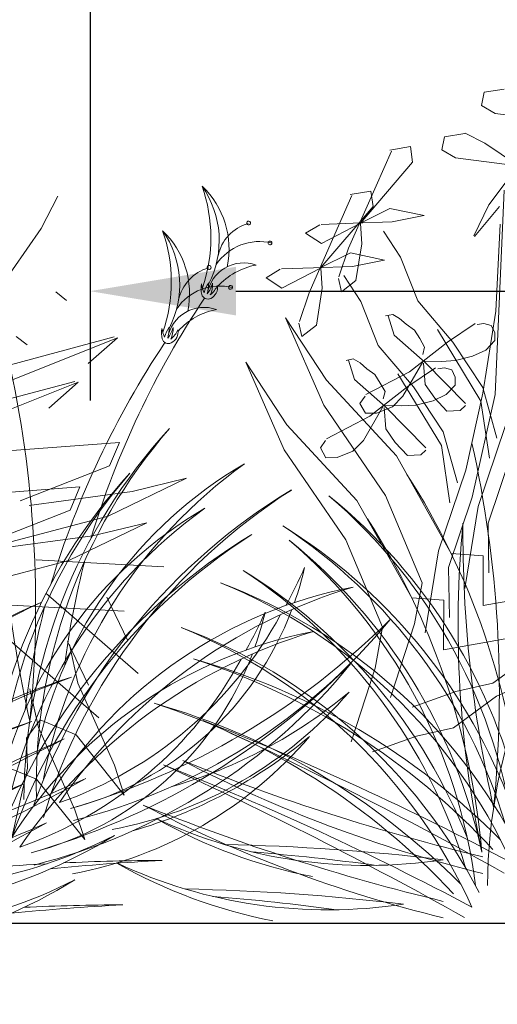
# Model space of a CAD drawing. Units: inches. Extents: x 89 to 490, y -59 to 378.
# Tile 5 of 20: x 326 to 339, y -26 to 1. Entities that reach past the tile are written whole.
import ezdxf

# ---------------------------------------------------------------- set-up
doc = ezdxf.new("R2010")
doc.units = ezdxf.units.IN
doc.header["$MEASUREMENT"] = 0
for name, color, linetype, lineweight in [('A-ANNO-DIMS', 2, 'Continuous', 18), ('L-PLNT', 94, 'Continuous', 18), ('L-PLNT-EDGE', 31, 'Continuous', 25)]:
    doc.layers.add(name, color=color, linetype=linetype, lineweight=lineweight)
doc.layers.add('fl', color=73, linetype='Continuous', lineweight=9, true_color=0xa3d166)
doc.styles.get("Standard").update_dxf_attribs({"font": 'arial.ttf'})
doc.dimstyles.get("Standard").update_dxf_attribs({"dimtxt": 6, "dimasz": 4, "dimexe": 3, "dimexo": 3, "dimgap": 0.09, "dimtad": 0, "dimtih": 1, "dimtoh": 1, "dimdec": 1, "dimzin": 0, "dimdsep": 46, "dimlunit": 3, "dimtxsty": 'Standard', "dimcen": 0.09, "dimadec": 0, "dimazin": 0, "dimtfac": 1, "dimtdec": 1, "dimtofl": 0, "dimtmove": 0, "dimatfit": 3, "dimfxl": 1, "dimtolj": 1, "dimtzin": 0, "dimarcsym": 0})

# ---------------------------------------------------------------- blocks, each defined once
blk = doc.blocks.new('Plantation')
at = {"layer": 'fl'}
for p, q in [((562.897, 34.348), (562.341, 34.259)), ((562.341, 34.259), (562.268, 33.899)), ((562.268, 33.899), (562.643, 33.679)), ((562.643, 33.679), (564.267, 33.469)), ((561.257, 33.041), (561.184, 32.681)), ((561.813, 33.13), (561.257, 33.041)), ((561.819, 33.139), (562.363, 32.866)), ((559.759, 32.671), (560.323, 32.769)), ((560.323, 32.769), (560.381, 32.343)), ((561.184, 32.681), (561.559, 32.461)), ((562.363, 32.866), (563.259, 32.265)), ((559.17, 31.216), (559.802, 32.648)), ((561.559, 32.461), (563.183, 32.251)), ((562.47, 31.169), (563.4, 32.416)), ((560.381, 32.343), (558.952, 30.67)), ((562.894, 31.579), (562.65, 25.971)), ((550.656, 31.412), (550.2, 30.521)), ((558.086, 29.998), (558.718, 31.43)), ((558.675, 31.453), (559.239, 31.551)), ((559.239, 31.551), (559.297, 31.125)), ((559.297, 31.125), (557.868, 29.452)), ((558.629, 29.982), (559.17, 31.216)), ((559.762, 31.074), (558.915, 30.657)), ((560.695, 30.877), (559.762, 31.074)), ((562.061, 30.328), (562.47, 31.169)), ((562.075, 30.305), (562.765, 31.127)), ((559.819, 30.704), (560.688, 30.879)), ((550.2, 30.521), (548.393, 27.932)), ((557.835, 30.626), (557.449, 30.393)), ((557.877, 30.637), (558.751, 30.667)), ((557.881, 30.111), (558.94, 30.658)), ((558.751, 30.667), (559.819, 30.704)), ((558.987, 30.105), (558.952, 30.658)), ((562.666, 28.259), (562.78, 30.644)), ((557.449, 30.393), (557.881, 30.111)), ((559.585, 30.453), (560.047, 29.739)), ((557.545, 28.764), (558.086, 29.998)), ((558.364, 29.196), (558.629, 29.982)), ((558.829, 29.096), (558.987, 30.105)), ((558.678, 29.856), (557.831, 29.439)), ((559.611, 29.659), (558.678, 29.856)), ((560.047, 29.739), (560.525, 28.54)), ((556.793, 29.419), (557.667, 29.449)), ((556.798, 28.893), (557.856, 29.44)), ((557.667, 29.449), (558.736, 29.486)), ((557.903, 28.887), (557.869, 29.44)), ((558.736, 29.486), (559.605, 29.661)), ((556.751, 29.408), (556.365, 29.175)), ((556.365, 29.175), (556.798, 28.893)), ((558.35, 29.151), (558.432, 28.787)), ((558.501, 29.235), (558.963, 28.521)), ((557.745, 27.878), (557.903, 28.887)), ((558.432, 28.787), (558.829, 29.096)), ((550.6, 28.785), (550.899, 28.552)), ((557.28, 27.978), (557.545, 28.764)), ((558.963, 28.521), (559.441, 27.322)), ((560.525, 28.54), (561.487, 27.406)), ((557.949, 25.681), (556.895, 28.076)), ((556.895, 28.076), (558.023, 26.364)), ((559.642, 28.128), (559.841, 28.168)), ((559.709, 28.134), (559.873, 27.605)), ((559.841, 28.168), (560.025, 28.061)), ((562.306, 26.01), (562.666, 28.259)), ((557.267, 27.933), (557.348, 27.569)), ((557.348, 27.569), (557.745, 27.878)), ((560.025, 28.061), (560.21, 27.901)), ((560.21, 27.901), (560.431, 27.741)), ((561.338, 27.412), (562.098, 27.924)), ((562.338, 27.92), (562.156, 27.898)), ((562.539, 27.869), (562.338, 27.92)), ((562.633, 27.67), (562.539, 27.869)), ((552.203, 27.553), (546.246, 25.952)), ((548.842, 26.149), (552.295, 27.53)), ((549.516, 27.567), (549.816, 27.334)), ((552.295, 27.53), (551.493, 26.822)), ((559.873, 27.605), (560.725, 26.856)), ((560.431, 27.741), (560.58, 27.507)), ((561.061, 27.757), (562.256, 25.796)), ((562.637, 27.452), (562.633, 27.67)), ((559.441, 27.322), (560.404, 26.188)), ((560.296, 26.598), (561.338, 27.412)), ((560.58, 27.507), (560.712, 27.272)), ((560.712, 27.272), (560.661, 27.071)), ((561.487, 27.406), (562.307, 26.17)), ((562.387, 27.192), (562.637, 27.452)), ((561.555, 26.905), (562.026, 27.022)), ((562.026, 27.022), (562.387, 27.192)), ((556.865, 24.463), (555.811, 26.858)), ((555.811, 26.858), (556.939, 25.146)), ((558.558, 26.91), (558.757, 26.949)), ((558.625, 26.916), (558.789, 26.387)), ((558.757, 26.949), (558.941, 26.843)), ((558.941, 26.843), (559.126, 26.683)), ((560.117, 25.933), (560.664, 26.871)), ((560.683, 26.835), (560.73, 26.253)), ((560.718, 26.89), (561.173, 26.88)), ((560.725, 26.856), (561.833, 25.727)), ((561.173, 26.88), (561.555, 26.905)), ((559.102, 25.974), (560.296, 26.598)), ((559.126, 26.683), (559.347, 26.523)), ((559.347, 26.523), (559.496, 26.289)), ((559.977, 26.539), (561.172, 24.578)), ((560.254, 26.194), (561.014, 26.706)), ((561.254, 26.702), (561.072, 26.68)), ((561.455, 26.651), (561.254, 26.702)), ((561.549, 26.452), (561.455, 26.651)), ((561.553, 26.234), (561.549, 26.452)), ((551.119, 26.335), (545.162, 24.734)), ((547.759, 24.931), (551.212, 26.312)), ((551.212, 26.312), (550.409, 25.604)), ((558.023, 26.364), (559.941, 24.291)), ((558.789, 26.387), (559.641, 25.638)), ((559.212, 25.38), (560.254, 26.194)), ((559.496, 26.289), (559.628, 26.054)), ((560.404, 26.188), (561.224, 24.952)), ((560.73, 26.253), (560.991, 25.875)), ((561.303, 25.974), (561.553, 26.234)), ((559.08, 25.933), (558.938, 25.73)), ((559.628, 26.054), (559.577, 25.853)), ((559.831, 25.636), (560.117, 25.933)), ((560.942, 25.804), (561.303, 25.974)), ((561.843, 23.904), (562.306, 26.01)), ((562.65, 25.971), (562.016, 23.158)), ((562.307, 26.17), (562.695, 24.774)), ((559.637, 23.211), (557.949, 25.681)), ((558.938, 25.73), (559.088, 25.459)), ((559.033, 24.715), (559.58, 25.653)), ((559.635, 25.672), (560.09, 25.662)), ((559.641, 25.638), (560.749, 24.509)), ((560.09, 25.662), (560.471, 25.687)), ((560.471, 25.687), (560.942, 25.804)), ((560.991, 25.875), (561.325, 25.517)), ((561.688, 25.541), (561.831, 25.671)), ((562.256, 25.796), (562.488, 24.228)), ((558.018, 24.756), (559.212, 25.38)), ((559.088, 25.459), (559.397, 25.465)), ((559.397, 25.465), (559.831, 25.636)), ((559.599, 25.617), (559.646, 25.035)), ((561.325, 25.517), (561.688, 25.541)), ((556.939, 25.146), (558.857, 23.073)), ((562.176, 22.909), (562.927, 25.122)), ((559.646, 25.035), (559.907, 24.657)), ((561.224, 24.952), (561.611, 23.556)), ((548.902, 24.401), (552.345, 24.664)), ((552.345, 24.664), (552.075, 24.023)), ((557.996, 24.715), (557.854, 24.512)), ((558.747, 24.418), (559.033, 24.715)), ((559.907, 24.657), (560.241, 24.299)), ((561.172, 24.578), (561.404, 23.01)), ((558.554, 21.993), (556.865, 24.463)), ((557.854, 24.512), (558.004, 24.241)), ((558.313, 24.247), (558.747, 24.418)), ((559.941, 24.291), (561.442, 21.62)), ((560.241, 24.299), (560.604, 24.323)), ((560.604, 24.323), (560.747, 24.453)), ((563.1, 24.376), (562.451, 22.451)), ((552.075, 24.023), (549.628, 23.064)), ((558.004, 24.241), (558.313, 24.247)), ((561.092, 21.691), (561.843, 23.904)), ((554.182, 23.678), (552.039, 22.642)), ((552.692, 23.319), (554.182, 23.678)), ((547.818, 23.183), (551.261, 23.446)), ((549.873, 22.937), (552.692, 23.319)), ((551.261, 23.446), (550.991, 22.805)), ((560.643, 20.815), (559.637, 23.211)), ((558.857, 23.073), (560.358, 20.402)), ((562.016, 23.158), (561.367, 21.233)), ((550.991, 22.805), (548.544, 21.846)), ((561.815, 20.66), (562.176, 22.909)), ((552.039, 22.642), (548.978, 21.84)), ((553.099, 22.46), (550.955, 21.424)), ((551.609, 22.101), (553.099, 22.46)), ((562.451, 22.451), (562.475, 21.085)), ((548.789, 21.719), (551.609, 22.101)), ((559.559, 19.597), (558.554, 21.993)), ((560.731, 19.442), (561.092, 21.691)), ((561.442, 21.62), (562.319, 21.552)), ((550.955, 21.424), (547.894, 20.622)), ((550.065, 21.443), (553.56, 21.255)), ((562.319, 21.552), (562.317, 20.191)), ((561.367, 21.233), (561.391, 19.867)), ((560.438, 19.69), (560.643, 20.815)), ((550.33, 20.533), (552.863, 18.331)), ((552.003, 20.423), (552.579, 19.227)), ((560.358, 20.402), (561.235, 20.334)), ((561.235, 20.334), (561.233, 18.973)), ((562.317, 20.191), (564.008, 20.492)), ((548.981, 20.225), (552.476, 20.037)), ((559.354, 18.472), (559.559, 19.597)), ((559.778, 17.674), (560.438, 19.69)), ((549.247, 19.315), (551.779, 17.113)), ((550.919, 19.205), (551.495, 18.009)), ((561.233, 18.973), (562.924, 19.274)), ((550.978, 19.124), (551.209, 18.062)), ((563.77, 18.928), (562.584, 18.061)), ((558.694, 16.456), (559.354, 18.472)), ((563.979, 18.289), (562.686, 17.71)), ((549.894, 17.906), (550.125, 16.844)), ((551.209, 18.062), (552.209, 15.812)), ((561.571, 17.832), (560.37, 17.403)), ((562.584, 18.061), (561.571, 17.832)), ((562.686, 17.71), (561.5, 16.843)), ((550.173, 17.055), (549.802, 16.556)), ((551.159, 16.651), (550.173, 17.055)), ((550.125, 16.844), (551.125, 14.594)), ((561.5, 16.843), (560.487, 16.614)), ((549.802, 16.556), (549.83, 15.731)), ((552.48, 14.995), (551.159, 16.651)), ((560.487, 16.614), (559.286, 16.185)), ((550.076, 15.433), (549.09, 15.837)), ((549.83, 15.731), (549.407, 13.869)), ((552.209, 15.812), (552.48, 14.995)), ((551.396, 13.777), (550.076, 15.433)), ((551.125, 14.594), (551.396, 13.777))]:
    blk.add_line(p, q, dxfattribs=at)
for centre, radius, start, end in [((552.48, 30.194), 2.601, 332.7126, 34.904), ((552.977, 29.961), 2.375, 348.2707, 46.4368), ((550.625, 30.285), 4.227, 340.8803, 19.3142), ((556.189, 29.542), 1.163, 105.8563, 168.2872), ((555.888, 30.675), 0.053, 350.198, 170.198), ((555.888, 30.675), 0.053, 170.198, 350.198), ((551.397, 28.976), 2.601, 332.7126, 34.904), ((551.893, 28.743), 2.375, 348.2707, 46.4368), ((549.541, 29.067), 4.227, 340.8803, 19.3142), ((556.176, 28.751), 1.416, 75.596, 146.3364), ((556.475, 30.129), 0.053, 170.198, 350.198), ((556.475, 30.129), 0.053, 350.198, 170.198), ((555.105, 28.324), 1.163, 105.8563, 168.2872), ((554.804, 29.457), 0.053, 170.198, 350.198), ((555.749, 28.572), 1.01, 70.2507, 170.8138), ((554.804, 29.457), 0.053, 350.198, 170.198), ((556.439, 27.67), 1.886, 100.6373, 137.9791), ((555.092, 27.533), 1.416, 75.596, 146.3364), ((555.27, 28.88), 0.688, 169.5666, 193.8466), ((555.783, 29.238), 1.213, 191.1134, 202.9272), ((555.444, 28.567), 0.803, 144.0451, 165.6539), ((553.282, 29.091), 1.513, 346.3307, 357.9859), ((554.082, 29.253), 0.848, 322.2492, 344.6889), ((554.247, 28.991), 0.654, 334.2428, 3.277), ((554.403, 29.244), 0.689, 308.8656, 336.2578), ((554.704, 28.911), 0.334, 295.3934, 9.6219), ((555.392, 28.911), 0.053, 170.198, 350.198), ((555.392, 28.911), 0.053, 350.198, 170.198), ((575.206, 14.886), 24.696, 146.2244, 163.2125), ((554.769, 28.765), 0.175, 196.6761, 296.6412), ((554.666, 27.354), 1.01, 70.2507, 170.8138), ((555.355, 26.452), 1.886, 100.6373, 137.9791), ((554.36, 27.349), 0.803, 144.0451, 165.6539), ((552.198, 27.873), 1.513, 346.3307, 357.9859), ((552.998, 28.035), 0.848, 322.2492, 344.6889), ((553.163, 27.773), 0.654, 334.2428, 3.277), ((554.186, 27.662), 0.688, 169.5666, 193.8466), ((554.699, 28.02), 1.213, 191.1134, 202.9272), ((553.319, 28.026), 0.689, 308.8656, 336.2578), ((553.62, 27.693), 0.334, 295.3934, 9.6219), ((574.122, 13.668), 24.696, 146.2244, 163.2125), ((553.685, 27.547), 0.175, 196.6761, 296.6412), ((518.556, 20.16), 31.492, 354.2791, 12.5427), ((564.924, 14.77), 15.201, 137.4916, 179.6099), ((564.986, 15.26), 14.921, 139.0392, 181.297), ((583.037, 24.54), 33.989, 179.5471, 192.7817), ((531.269, 17.801), 31.492, 354.2791, 12.5427), ((561.844, 13.707), 12.017, 120.3536, 167.8423), ((563.873, 12.836), 13.856, 125.7805, 169.1581), ((563.84, 13.552), 15.201, 137.4916, 179.6099), ((563.902, 14.042), 14.921, 139.0392, 181.297), ((543.232, 12.838), 20.216, 5.151, 32.7872), ((565.668, 9.115), 16.642, 121.1471, 160.292), ((565.801, 9.672), 16.239, 122.567, 163.1344), ((548.387, 11.862), 14.921, 7.1968, 49.4547), ((548.521, 11.386), 15.201, 12.4122, 51.0023), ((560.76, 12.489), 12.017, 120.3536, 167.8423), ((562.789, 11.618), 13.856, 125.7805, 169.1581), ((577.637, 12.411), 15.201, 137.4916, 179.6099), ((542.148, 11.62), 20.216, 5.151, 32.7872), ((591.525, 19.645), 29.894, 174.6174, 191.9895), ((595.75, 22.181), 33.989, 179.5471, 192.7817), ((564.584, 7.897), 16.642, 121.1471, 160.292), ((564.717, 8.454), 16.239, 122.567, 163.1344), ((548.639, 9.896), 14.921, 16.8321, 56.7339), ((548.831, 9.441), 15.201, 21.5651, 58.2814), ((547.303, 10.644), 14.921, 7.1968, 49.4547), ((547.437, 10.168), 15.201, 12.4122, 51.0023), ((572.745, 15.833), 22.067, 165.3183, 172.932), ((547.555, 8.678), 14.921, 16.8321, 56.7339), ((547.747, 8.223), 15.201, 21.5651, 58.2814), ((545.552, 26.474), 12.977, 331.0459, 336.1667), ((548.768, 23.222), 8.88, 340.6151, 347.0426), ((549.776, 6.58), 15.201, 27.2807, 69.4256), ((549.5, 6.989), 14.921, 24.3637, 67.878), ((561.156, 8.288), 12.64, 100.96, 147.8088), ((563.04, 6.416), 14.911, 106.7083, 145.8338), ((556.056, 6.249), 15.201, 112.5744, 154.7193), ((556.319, 6.667), 14.921, 114.122, 157.6363), ((571.661, 14.615), 22.067, 165.3183, 172.932), ((548.768, 23.222), 8.88, 284.6053, 339.2893), ((544.468, 25.256), 12.977, 331.0459, 336.1667), ((547.685, 22.004), 8.88, 340.6151, 347.0426), ((547.063, 25.215), 11.042, 289.2472, 331.4766), ((545.293, 34.281), 20.466, 286.2137, 315.0057), ((547.119, 30.131), 16.324, 284.0723, 320.7861), ((560.073, 7.07), 12.64, 100.96, 147.8088), ((561.956, 5.198), 14.911, 106.7083, 145.8338), ((548.693, 5.362), 15.201, 27.2807, 69.4256), ((548.416, 5.771), 14.921, 24.3637, 67.878), ((545.979, 23.997), 11.042, 289.2472, 331.4766), ((547.685, 22.004), 8.88, 284.6053, 339.2893), ((549.158, 0.259), 19.194, 44.7494, 74.2143), ((548.536, 0.496), 19.147, 42.8064, 72.2288), ((544.209, 33.063), 20.466, 286.2137, 315.0057), ((546.035, 28.913), 16.324, 284.0723, 320.7861), ((556.894, -0.047), 19.194, 107.7857, 137.2506), ((557.508, 0.211), 19.147, 109.7712, 139.1936), ((550.032, 25.179), 11.325, 280.7497, 319.4803), ((550.168, 27.86), 13.137, 285.9859, 310.1616), ((548.075, -0.959), 19.194, 44.7494, 74.2143), ((547.452, -0.722), 19.147, 42.8064, 72.2288), ((555.811, -1.265), 19.194, 107.7857, 137.2506), ((556.424, -1.007), 19.147, 109.7712, 139.1936), ((510.112, -81.018), 107.696, 60.65352, 65.57668), ((524.246, -59.986), 82.807, 62.02355, 68.46556), ((583.894, -59.385), 82.807, 113.53444, 119.97645), ((598.754, -79.911), 107.696, 116.42332, 121.34648), ((548.948, 23.961), 11.325, 280.7497, 319.4803), ((549.084, 26.642), 13.137, 285.9859, 310.1616), ((571.044, 48.565), 36.77, 242.5259, 256.2554), ((576.031, 70.211), 58.541, 247.9781, 256.44), ((509.028, -82.236), 107.696, 60.65352, 65.57668), ((523.162, -61.204), 82.807, 62.02355, 68.46556), ((527.597, 68.925), 58.541, 285.56, 294.0219), ((533.336, 47.466), 36.77, 285.7446, 299.4741), ((582.81, -60.603), 82.807, 113.53444, 119.97645), ((597.67, -81.129), 107.696, 116.42332, 121.34648), ((569.961, 47.347), 36.77, 242.5259, 256.2554), ((574.947, 68.993), 58.541, 247.9781, 256.44), ((560.311, 26.553), 14.044, 240.3144, 259.0249), ((559.15, 26.772), 13.704, 244.9915, 278.6666), ((526.513, 67.707), 58.541, 285.56, 294.0219), ((532.252, 46.248), 36.77, 285.7446, 299.4741), ((545.984, 26.101), 13.704, 263.3334, 297.0085), ((544.831, 25.842), 14.044, 282.9751, 301.6856), ((554.028, -46.704), 60.356, 83.15791, 88.86091), ((551.195, -46.771), 60.398, 82.20958, 85.44376), ((553.666, -47.151), 60.356, 93.13909, 98.84209), ((556.5, -47.12), 60.398, 92.82762, 95.73925), ((553.666, -47.151), 60.356, 90.13814, 92.7056), ((559.227, 25.335), 14.044, 240.3144, 259.0249), ((558.066, 25.554), 13.704, 244.9915, 278.6666), ((544.9, 24.883), 13.704, 263.3334, 297.0085), ((543.747, 24.624), 14.044, 282.9751, 301.6856), ((552.944, -47.922), 60.356, 83.15791, 88.86091), ((550.111, -47.989), 60.398, 82.20958, 85.44376), ((555.417, -48.338), 60.398, 92.82762, 95.73925), ((552.583, -48.369), 60.356, 90.13814, 92.7056)]:
    blk.add_arc(centre, radius, start, end, dxfattribs=at)
blk = doc.blocks.new('*D36')
at = {"layer": 'A-ANNO-DIMS', "color": 0, "lineweight": -2, "transparency": 16777216}
for p, q in [((327.654, 1.741), (327.654, -9.059)), ((399.654, 1.741), (399.654, -9.059)), ((331.654, -6.059), (339.621, -6.059)), ((395.654, -6.059), (387.687, -6.059))]:
    blk.add_line(p, q, dxfattribs=at)
at = {"layer": 'A-ANNO-DIMS', "color": 0, "transparency": 16777216}
for points in [[(331.654, -5.392), (331.654, -6.725), (327.654, -6.059)], [(395.654, -5.392), (395.654, -6.725), (399.654, -6.059)]]:
    blk.add_solid(points, dxfattribs=at)
at = {"layer": 'Defpoints', "color": 0, "transparency": 16777216}
for p in [(327.654, 4.741), (399.654, 4.741), (399.654, -6.059)]:
    blk.add_point(p, dxfattribs=at)
at = {"layer": 'A-ANNO-DIMS', "color": 0, "transparency": 16777216, "insert": (363.654, -6.059), "char_height": 6, "attachment_point": 5}
blk.add_mtext('\\A1;WINDOW 72', dxfattribs=at)
blk = doc.blocks.new('*D46')
at = {"layer": 'A-ANNO-DIMS', "color": 0, "lineweight": -2, "transparency": 16777216}
for p, q in [((277.443, -27.866), (277.443, -53.11)), ((445.739, -27.866), (445.739, -53.11)), ((281.443, -50.11), (332.892, -50.11)), ((441.739, -50.11), (390.289, -50.11))]:
    blk.add_line(p, q, dxfattribs=at)
at = {"layer": 'A-ANNO-DIMS', "color": 0, "transparency": 16777216}
for points in [[(281.443, -49.443), (281.443, -50.777), (277.443, -50.11)], [(441.739, -49.443), (441.739, -50.777), (445.739, -50.11)]]:
    blk.add_solid(points, dxfattribs=at)
at = {"layer": 'Defpoints', "color": 0, "transparency": 16777216}
for p in [(277.443, -24.866), (445.739, -24.866), (445.739, -50.11)]:
    blk.add_point(p, dxfattribs=at)
at = {"layer": 'A-ANNO-DIMS', "color": 0, "transparency": 16777216, "insert": (361.591, -50.11), "char_height": 6, "attachment_point": 5}
blk.add_mtext('\\A1;PLANTING 168', dxfattribs=at)
blk = doc.blocks.new('*D48')
at = {"layer": 'A-ANNO-DIMS', "color": 0, "lineweight": -2, "transparency": 16777216}
for p, q in [((127.441, 10.741), (127.441, -49.809)), ((459.441, -29.659), (459.441, -49.809)), ((131.441, -46.809), (286.756, -46.809)), ((455.441, -46.809), (300.127, -46.809))]:
    blk.add_line(p, q, dxfattribs=at)
at = {"layer": 'A-ANNO-DIMS', "color": 0, "transparency": 16777216}
for points in [[(131.441, -46.143), (131.441, -47.476), (127.441, -46.809)], [(455.441, -46.143), (455.441, -47.476), (459.441, -46.809)]]:
    blk.add_solid(points, dxfattribs=at)
at = {"layer": 'Defpoints', "color": 0, "transparency": 16777216}
for p in [(127.441, 13.741), (459.441, -26.659), (459.441, -46.809)]:
    blk.add_point(p, dxfattribs=at)
at = {"layer": 'A-ANNO-DIMS', "color": 0, "transparency": 16777216, "insert": (293.441, -46.809), "char_height": 6, "attachment_point": 5}
blk.add_mtext('\\A1;332', dxfattribs=at)

msp = doc.modelspace()

# ---------------------------------------------------------------- linework, layer by layer
at = {"layer": 'L-PLNT-EDGE'}
msp.add_line((459.4414, -23.3886), (265.4414, -23.3886), dxfattribs=at)

# ---------------------------------------------------------------- block references
at = {"layer": 'L-PLNT'}
msp.add_blockref('Plantation', (-223.8856, -34.8668), dxfattribs=at)

# ---------------------------------------------------------------- dimensions: what is measured, and where the dimension line sits
at = {"layer": 'A-ANNO-DIMS'}
dim = msp.add_linear_dim(base=(459.4414, -46.8094), p1=(127.4414, 13.7413), p2=(459.4414, -26.6594), dimstyle='Standard', override={"dimdec": 0, "dimlfac": 1, "dimrnd": 0, "dimzin": 0, "dimdsep": 46, "dimlunit": 2}, dxfattribs=at)
dim.commit()
dim.dimension.update_dxf_attribs({"geometry": '*D48', "text_midpoint": (293.4414, -46.8094)})
for base, p1, p2, text, picture, middle in [((399.6539, -6.0587), (327.6539, 4.7413), (399.6539, 4.7413), 'WINDOW <>', '*D36', (363.6539, -6.0587)), ((445.7386, -50.11), (277.443, -24.8656), (445.7386, -24.8656), 'PLANTING <>', '*D46', (361.5908, -50.11))]:
    dim = msp.add_linear_dim(base=base, p1=p1, p2=p2, text=text, dimstyle='Standard', override={"dimdec": 0, "dimlfac": 1, "dimrnd": 0, "dimzin": 0, "dimdsep": 46, "dimlunit": 2}, dxfattribs=at)
    dim.commit()
    dim.dimension.update_dxf_attribs({"geometry": picture, "text_midpoint": middle})

doc.saveas('drawing.dxf')
